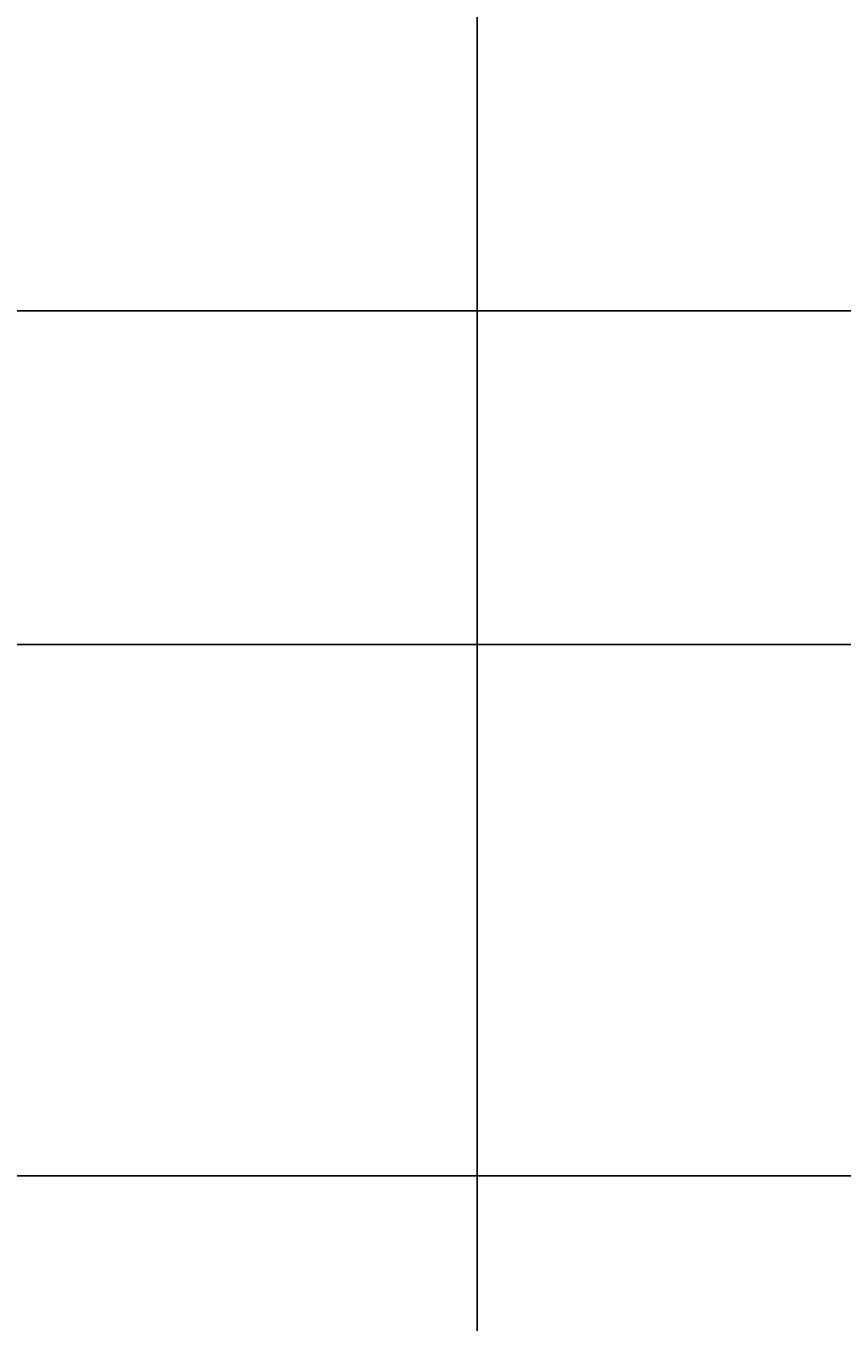
# Model space of a CAD drawing. Units: inches. Extents: x 35362 to 73946, y 43607 to 67532.
# Tile 58 of 134: x 51337 to 52380, y 45263 to 46919. Entities that reach past the tile are written whole.
import ezdxf

# ---------------------------------------------------------------- set-up
doc = ezdxf.new("R2010")
doc.units = ezdxf.units.IN
doc.header["$MEASUREMENT"] = 0
doc.layers.add('A-ANNO-DIMS', color=2, linetype='Continuous', lineweight=18)
doc.styles.get("Standard").update_dxf_attribs({"font": 'arial.ttf'})
doc.dimstyles.get("Standard").update_dxf_attribs({"dimtxt": 0.18, "dimasz": 0.18, "dimexe": 0.18, "dimexo": 0.0625, "dimgap": 0.09, "dimtad": 0, "dimtih": 1, "dimtoh": 1, "dimdec": 4, "dimzin": 0, "dimdsep": 46, "dimtxsty": 'Standard', "dimcen": 0.09, "dimadec": 0, "dimazin": 0, "dimtfac": 1, "dimtdec": 4, "dimtofl": 0, "dimtmove": 0, "dimatfit": 3, "dimfxl": 1, "dimtolj": 1, "dimtzin": 0, "dimarcsym": 0})

# ---------------------------------------------------------------- blocks, each defined once
blk = doc.blocks.new('*D5')
at = {"layer": 'A-ANNO-DIMS', "color": 0, "lineweight": -2, "transparency": 16777216}
for p, q in [((37121.9, 46919.3), (37121.9, 43606.7)), ((69871.5, 45449.8), (69871.5, 43606.7)), ((37122.1, 43606.9), (53496.3, 43606.9)), ((69871.3, 43606.9), (53497.2, 43606.9))]:
    blk.add_line(p, q, dxfattribs=at)
at = {"layer": 'A-ANNO-DIMS', "color": 0, "transparency": 16777216}
for points in [[(37122.1, 43606.9), (37122.1, 43606.8), (37121.9, 43606.9)], [(69871.3, 43606.9), (69871.3, 43606.8), (69871.5, 43606.9)]]:
    blk.add_solid(points, dxfattribs=at)
at = {"layer": 'Defpoints', "color": 0, "transparency": 16777216}
for p in [(37121.9, 46919.4), (69871.5, 45449.9), (69871.5, 43606.9)]:
    blk.add_point(p, dxfattribs=at)
at = {"layer": 'A-ANNO-DIMS', "color": 0, "transparency": 16777216, "insert": (53496.7, 43606.9), "char_height": 0.18, "attachment_point": 5}
blk.add_mtext('\\A1;32750', dxfattribs=at)
blk = doc.blocks.new('*D11')
at = {"layer": 'A-ANNO-DIMS', "color": 0, "lineweight": -2, "transparency": 16777216}
for p, q in [((47978.7, 56028.8), (47978.7, 43606.7)), ((53109.8, 56028.8), (53109.8, 43606.7)), ((47978.8, 43606.9), (50543.9, 43606.9)), ((53109.6, 43606.9), (50544.6, 43606.9))]:
    blk.add_line(p, q, dxfattribs=at)
at = {"layer": 'A-ANNO-DIMS', "color": 0, "transparency": 16777216}
for points in [[(47978.8, 43606.9), (47978.8, 43606.8), (47978.7, 43606.9)], [(53109.6, 43606.9), (53109.6, 43606.8), (53109.8, 43606.9)]]:
    blk.add_solid(points, dxfattribs=at)
at = {"layer": 'Defpoints', "color": 0, "transparency": 16777216}
for p in [(47978.7, 56028.8), (53109.8, 56028.8), (53109.8, 43606.9)]:
    blk.add_point(p, dxfattribs=at)
at = {"layer": 'A-ANNO-DIMS', "color": 0, "transparency": 16777216, "insert": (50544.2, 43606.9), "char_height": 0.18, "attachment_point": 5}
blk.add_mtext('\\A1;5131', dxfattribs=at)
blk = doc.blocks.new('*D17')
at = {"layer": 'A-ANNO-DIMS', "color": 0, "lineweight": -2, "transparency": 16777216}
for p, q in [((49923.3, 61293.2), (49923.3, 43606.7)), ((51913.9, 61293.2), (51913.9, 43606.7)), ((49923.5, 43606.9), (50918.2, 43606.9)), ((51913.8, 43606.9), (50919.1, 43606.9))]:
    blk.add_line(p, q, dxfattribs=at)
at = {"layer": 'A-ANNO-DIMS', "color": 0, "transparency": 16777216}
for points in [[(49923.5, 43606.9), (49923.5, 43606.8), (49923.3, 43606.9)], [(51913.8, 43606.9), (51913.8, 43606.8), (51913.9, 43606.9)]]:
    blk.add_solid(points, dxfattribs=at)
at = {"layer": 'Defpoints', "color": 0, "transparency": 16777216}
for p in [(49923.3, 61293.3), (51913.9, 61293.3), (51913.9, 43606.9)]:
    blk.add_point(p, dxfattribs=at)
at = {"layer": 'A-ANNO-DIMS', "color": 0, "transparency": 16777216, "insert": (50918.6, 43606.9), "char_height": 0.18, "attachment_point": 5}
blk.add_mtext('\\A1;1990.6', dxfattribs=at)
blk = doc.blocks.new('*D67')
at = {"layer": 'A-ANNO-DIMS', "color": 0, "lineweight": -2, "transparency": 16777216}
for p, q in [((56873.5, 53351.5), (35361.8, 53351.5)), ((35361.9, 53351.3), (35361.9, 49400.9)), ((35361.9, 45450.1), (35361.9, 49400.5)), ((53793.6, 45449.9), (35361.8, 45449.9))]:
    blk.add_line(p, q, dxfattribs=at)
at = {"layer": 'A-ANNO-DIMS', "color": 0, "transparency": 16777216}
for points in [[(35361.9, 53351.3), (35362, 53351.3), (35361.9, 53351.5)], [(35361.9, 45450.1), (35362, 45450.1), (35361.9, 45449.9)]]:
    blk.add_solid(points, dxfattribs=at)
at = {"layer": 'Defpoints', "color": 0, "transparency": 16777216}
for p in [(35361.9, 53351.5), (56873.6, 53351.5), (53793.6, 45449.9)]:
    blk.add_point(p, dxfattribs=at)
at = {"layer": 'A-ANNO-DIMS', "color": 0, "transparency": 16777216, "insert": (35361.9, 49400.7), "char_height": 0.18, "attachment_point": 5}
blk.add_mtext('\\A1;7901.6', dxfattribs=at)
blk = doc.blocks.new('*D76')
at = {"layer": 'A-ANNO-DIMS', "color": 0, "lineweight": -2, "transparency": 16777216}
for p, q in [((54052.8, 46555.3), (35361.8, 46555.3)), ((35361.9, 46555.1), (35361.9, 46342.3)), ((35361.9, 46129.1), (35361.9, 46341.9)), ((53793.6, 46128.9), (35361.8, 46128.9))]:
    blk.add_line(p, q, dxfattribs=at)
at = {"layer": 'A-ANNO-DIMS', "color": 0, "transparency": 16777216}
for points in [[(35361.9, 46555.1), (35362, 46555.1), (35361.9, 46555.3)], [(35361.9, 46129.1), (35362, 46129.1), (35361.9, 46128.9)]]:
    blk.add_solid(points, dxfattribs=at)
at = {"layer": 'Defpoints', "color": 0, "transparency": 16777216}
for p in [(35361.9, 46555.3), (54052.9, 46555.3), (53793.6, 46128.9)]:
    blk.add_point(p, dxfattribs=at)
at = {"layer": 'A-ANNO-DIMS', "color": 0, "transparency": 16777216, "insert": (35361.9, 46342.1), "char_height": 0.18, "attachment_point": 5}
blk.add_mtext('\\A1;426.4', dxfattribs=at)
blk = doc.blocks.new('*D90')
at = {"layer": 'A-ANNO-DIMS', "color": 0, "lineweight": -2, "transparency": 16777216}
for p, q in [((53707.7, 47291.3), (35361.8, 47291.3)), ((35361.9, 47291.1), (35361.9, 46710.3)), ((35361.9, 46129.1), (35361.9, 46709.9)), ((53793.6, 46128.9), (35361.8, 46128.9))]:
    blk.add_line(p, q, dxfattribs=at)
at = {"layer": 'A-ANNO-DIMS', "color": 0, "transparency": 16777216}
for points in [[(35361.9, 47291.1), (35362, 47291.1), (35361.9, 47291.3)], [(35361.9, 46129.1), (35362, 46129.1), (35361.9, 46128.9)]]:
    blk.add_solid(points, dxfattribs=at)
at = {"layer": 'Defpoints', "color": 0, "transparency": 16777216}
for p in [(53707.8, 47291.3), (35361.9, 46128.9), (53793.6, 46128.9)]:
    blk.add_point(p, dxfattribs=at)
at = {"layer": 'A-ANNO-DIMS', "color": 0, "transparency": 16777216, "insert": (35361.9, 46710.1), "char_height": 0.18, "attachment_point": 5}
blk.add_mtext('\\A1;1162.4', dxfattribs=at)

msp = doc.modelspace()

# ---------------------------------------------------------------- dimensions: what is measured, and where the dimension line sits
at = {"layer": 'A-ANNO-DIMS'}
for base, p1, p2, override, picture, middle in [((51913.931, 43606.859), (49923.307, 61293.286), (51913.931, 61293.286), {"dimdec": 1, "dimlfac": 1, "dimrnd": 0, "dimzin": 0, "dimdsep": 46, "dimlunit": 2}, '*D17', (50918.619, 43606.859)), ((53109.76, 43606.859), (47978.665, 56028.836), (53109.76, 56028.836), {"dimdec": 0, "dimlfac": 1, "dimrnd": 0, "dimzin": 0, "dimdsep": 46, "dimlunit": 2}, '*D11', (50544.212, 43606.859)), ((69871.496, 43606.859), (37121.949, 46919.381), (69871.496, 45449.894), {"dimdec": 0, "dimlfac": 1, "dimrnd": 0, "dimzin": 0, "dimdsep": 46, "dimlunit": 2}, '*D5', (53496.723, 43606.859))]:
    dim = msp.add_linear_dim(base=base, p1=p1, p2=p2, dimstyle='Standard', override=override, dxfattribs=at)
    dim.commit()
    dim.dimension.update_dxf_attribs({"geometry": picture, "text_midpoint": middle})
for base, p1, p2, picture, middle in [((35361.949, 53351.529), (53793.638, 45449.894), (56873.602, 53351.529), '*D67', (35361.949, 49400.712)), ((35361.949, 46128.878), (53707.781, 47291.285), (53793.638, 46128.878), '*D90', (35361.949, 46710.081)), ((35361.949, 46555.293), (53793.638, 46128.878), (54052.899, 46555.293), '*D76', (35361.949, 46342.086))]:
    dim = msp.add_linear_dim(base=base, p1=p1, p2=p2, angle=90, dimstyle='Standard', override={"dimdec": 1, "dimlfac": 1, "dimrnd": 0, "dimzin": 0, "dimdsep": 46, "dimlunit": 2}, dxfattribs=at)
    dim.commit()
    dim.dimension.update_dxf_attribs({"geometry": picture, "text_midpoint": middle})

doc.saveas('drawing.dxf')
